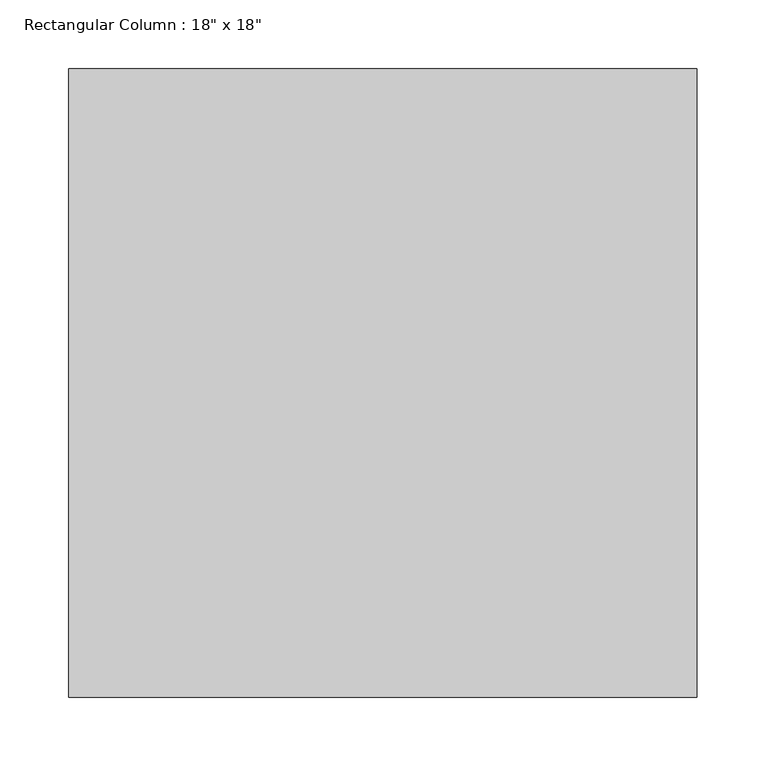
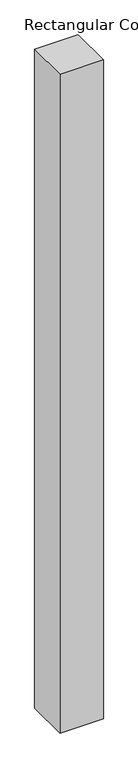
"""IFC4 building model written with IfcOpenShell, lengths in millimetres: column geometry."""

from ifc_helpers import new_model, si_unit, origin, origin_with_axes, place, context, project, spatial, polyline, outline, extrude, source, transform, mapped, element, save


def column_b90849dc(model_context):
    return source(origin(), model_context, "Body", "SweptSolid", [
        extrude(outline(polyline([(228.6, 228.6), (228.6, -228.6), (-228.6, -228.6), (-228.6, 228.6), (228.6, 228.6)])), origin_with_axes(), (0.0, 0.0, 1.0), 7315.2),
    ])


if __name__ == "__main__":
    model = new_model("IFC4")
    model_context = context("Model", 3, world=origin())
    ifc_project = project(units=[si_unit("LENGTHUNIT", "METRE", prefix="MILLI")], contexts=[model_context])
    site = spatial("IfcSite", under=ifc_project)
    building = spatial("IfcBuilding", under=site)
    placement = place(None, origin())
    column_shape = column_b90849dc(model_context)
    element("IfcColumn", 1, ObjectType="Rectangular Column : 18\" x 18\"", at=placement, inside=building, context=model_context, shape_type="MappedRepresentation", body=[
        mapped(column_shape, transform((0.0, 0.0, 0.0), x_axis=(1.0, 0.0, 0.0), y_axis=(0.0, 1.0, 0.0), z_axis=(0.0, 0.0, 1.0))),
    ])
    save(model, "model.ifc")

# Revit data of these elements
# Type "Rectangular Column : 18\" x 18\""
#   Assembly Code = "B1010200"
#   Depth = 1' - 6"
#   Offset Base = 0' - 0"
#   Offset Top = 0' - 0"
#   Width = 1' - 6"
#   Material = none
